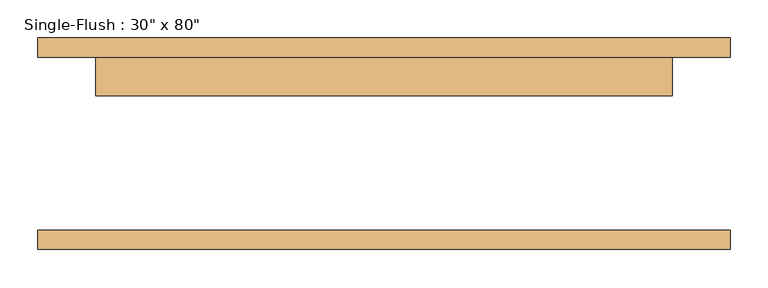
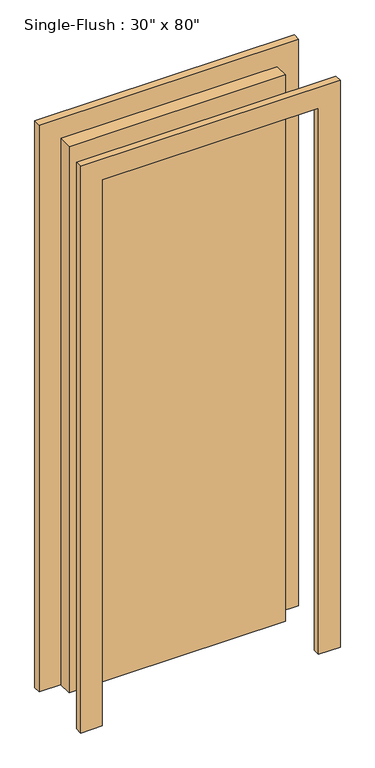
"""IFC4 building model written with IfcOpenShell, lengths in millimetres: door geometry."""

from ifc_helpers import new_model, si_unit, frame, origin, origin_with_axes, place, context, project, spatial, polyline, outline, extrude, source, transform, mapped, element, save


def door_a1484949(model_context):
    return source(origin(), model_context, "Body", "SweptSolid", [
        extrude(outline(polyline([(2108.2, -457.2), (0.0, -457.2), (0.0, -381.0), (2032.0, -381.0), (2032.0, 381.0), (0.0, 381.0), (0.0, 457.2), (2108.2, 457.2), (2108.2, -457.2)])), frame((0.0, 114.3, 0.0), z_axis=(0.0, 1.0, 0.0), x_axis=(0.0, 0.0, 1.0)), (0.0, 0.0, 1.0), 25.4),
        extrude(outline(polyline([(2108.2, 457.2), (2108.2, -457.2), (0.0, -457.2), (0.0, -381.0), (2032.0, -381.0), (2032.0, 381.0), (0.0, 381.0), (0.0, 457.2), (2108.2, 457.2)])), frame((0.0, -139.7, 0.0), z_axis=(0.0, 1.0, 0.0), x_axis=(0.0, 0.0, 1.0)), (0.0, 0.0, 1.0), 25.4),
        extrude(outline(polyline([(381.0, 63.5), (-381.0, 63.5), (-381.0, 114.3), (381.0, 114.3), (381.0, 63.5)])), origin_with_axes(), (0.0, 0.0, 1.0), 2032.0),
    ])


if __name__ == "__main__":
    model = new_model("IFC4")
    model_context = context("Model", 3, world=origin())
    ifc_project = project(units=[si_unit("LENGTHUNIT", "METRE", prefix="MILLI")], contexts=[model_context])
    site = spatial("IfcSite", under=ifc_project)
    building = spatial("IfcBuilding", under=site)
    placement = place(None, origin())
    door_shape = door_a1484949(model_context)
    element("IfcDoor", 1, ObjectType="Single-Flush : 30\" x 80\"", at=placement, inside=building, context=model_context, shape_type="MappedRepresentation", body=[
        mapped(door_shape, transform((0.0, 0.0, 0.0), x_axis=(1.0, 0.0, 0.0), y_axis=(0.0, 1.0, 0.0), z_axis=(0.0, 0.0, 1.0))),
    ])
    save(model, "model.ifc")

# Revit data of these elements
# Type "Single-Flush : 30\" x 80\""
#   Type Mark = "5"
#   Construction Type Id = "MDOOR"
#   Assembly Code = "C1020"
#   Analytic Construction = "Metal"
#   Thickness = 0' - 2"
#   Heat Transfer Coefficient (U) = 0.651978 BTU/(h·ft²·°F)
#   Height = 6' - 8"
#   Trim Projection Ext = 0' - 1"
#   Trim Projection Int = 0' - 1"
#   Trim Width = 0' - 3"
#   Width = 2' - 6"
#   Define Thermal Properties by = 1
#   Define Thermal Properties by = 1
#   Door Material = Door - Panel
#   Frame Material = Door - Frame
#   Visual Light Transmittance = 0
#   Solar Heat Gain Coefficient = 0
#   Function = (empty or 0)
#   Wall Closure = (empty or 0)
# Element 1 (IfcDoor, "Single-Flush : 30\" x 80\"")
#   Materials on its faces: "Door - Frame", "Door - Panel"
# Materials
#   "Door - Panel": class "Wood", colour RGB 210 159 95, transparency 0, Cost = 0
#   "Door - Frame": colour RGB 118 70 51, transparency 0, Cost = 0
